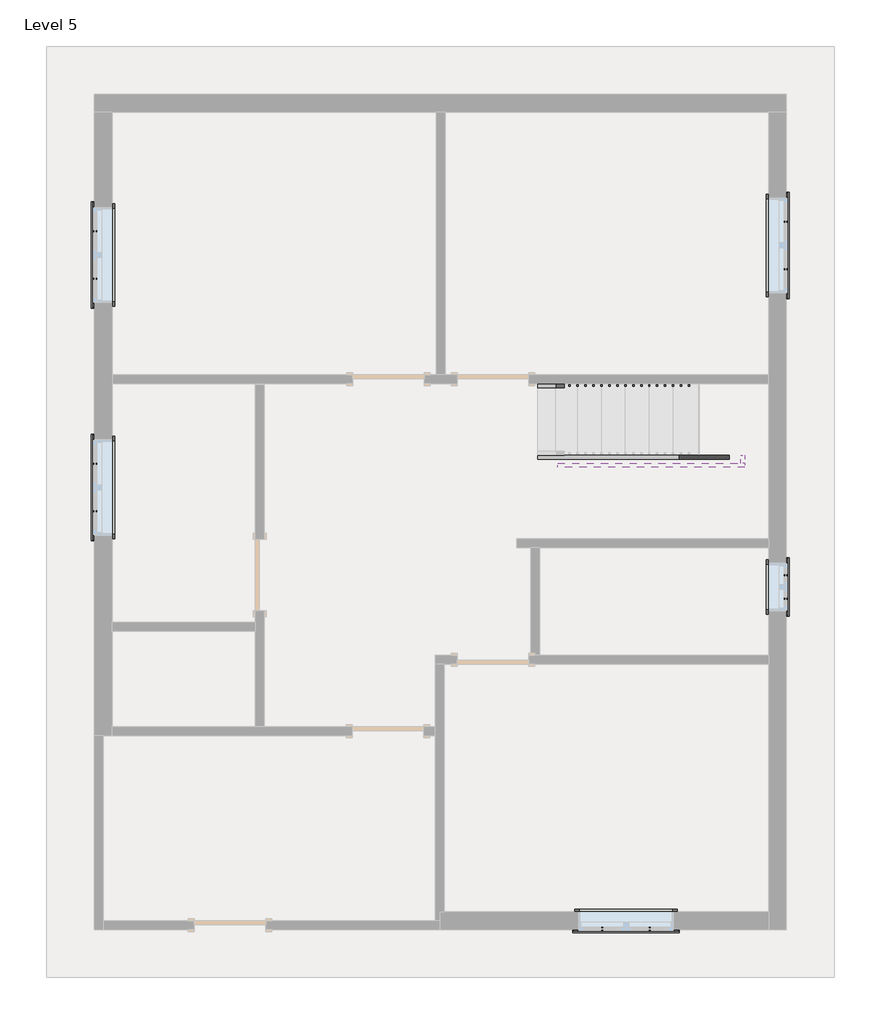
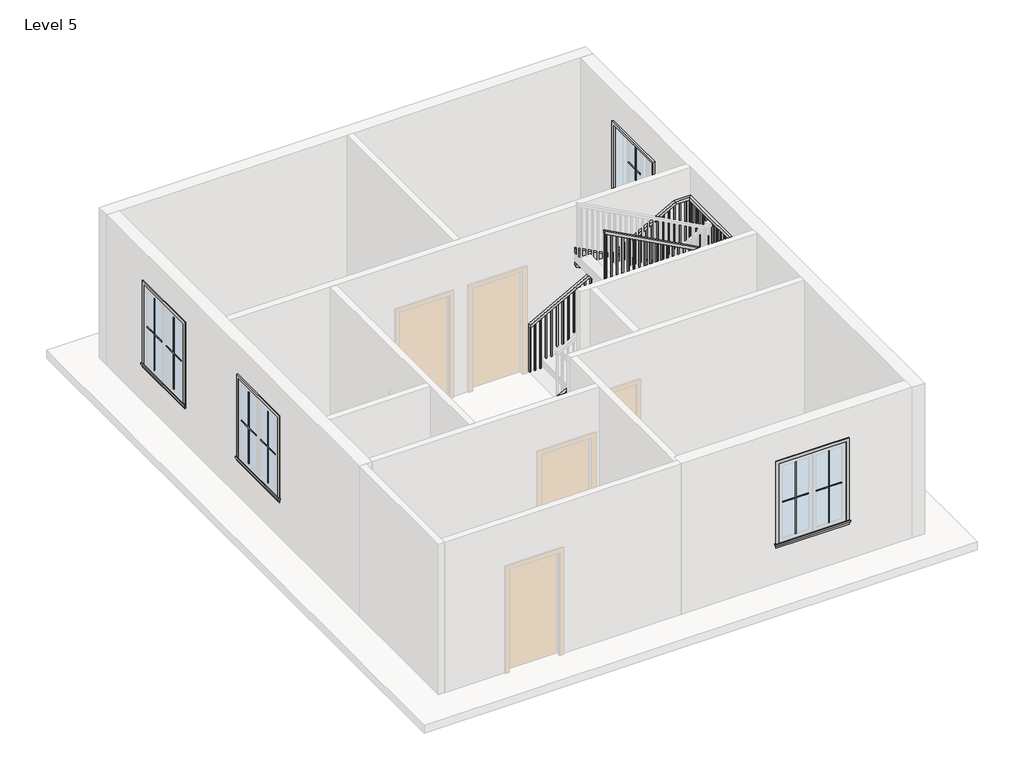
# One storey, part 2 of 2: 20 proxies, 3 members, 1 railing.
"""IFC4 building model written with IfcOpenShell, lengths in millimetres."""

from ifc_helpers import new_model, si_unit, frame, origin, place, context, project, spatial, polyline, outline, extrude, faceted_brep, transform, mapped, element, save
from components import muntin_pattern_2x2_muntin_pattern_2x2_6dad3731, muntin_pattern_2x2_muntin_pattern_2x2_a30a3345, muntin_pattern_2x2_muntin_pattern_2x2_53152e2c, muntin_pattern_2x2_muntin_pattern_2x2_e8f3e573, trim_window_exterior_flat_with_sill_92b9b949, trim_window_exterior_flat_with_sill_a665a915, trim_window_interior_flat_picture_frame_3bb882cf, trim_window_interior_flat_picture_frame_d485c387

model = new_model("IFC4")

# Units and contexts
model_context = context("Model", 3, world=origin())
ifc_project = project(units=[si_unit("LENGTHUNIT", "METRE", prefix="MILLI")], contexts=[model_context])

# Site, building, storey
site = spatial("IfcSite", under=ifc_project)
building = spatial("IfcBuilding", under=site)
storey = spatial("IfcBuildingStorey", under=building, Name="Level 5", Elevation=12192.0)

# Proxies
placement = place(None, origin())
muntin_pattern_2x2_muntin_pattern_2x2_shape = muntin_pattern_2x2_muntin_pattern_2x2_6dad3731(model_context)
element("IfcBuildingElementProxy", 1, Name="Muntin Pattern_2x2 : Muntin Pattern_2x2", ObjectType="Muntin Pattern_2x2 : Muntin Pattern_2x2", at=placement, inside=storey, context=model_context, shape_type="MappedRepresentation", body=[
    mapped(muntin_pattern_2x2_muntin_pattern_2x2_shape, transform((10003.63125, 2232.025, 13176.25), x_axis=(-1.0, 0.0, 0.0), y_axis=(0.0, -1.0, 0.0), z_axis=(0.0, 0.0, 1.0))),
])
element("IfcBuildingElementProxy", 2, Name="Muntin Pattern_2x2 : Muntin Pattern_2x2", ObjectType="Muntin Pattern_2x2 : Muntin Pattern_2x2", at=placement, inside=storey, context=model_context, shape_type="MappedRepresentation", body=[
    mapped(muntin_pattern_2x2_muntin_pattern_2x2_shape, transform((2917.825, 7567.6125, 13176.25), x_axis=(0.0, 1.0, 0.0), y_axis=(-1.0, 0.0, 0.0), z_axis=(0.0, 0.0, 1.0))),
])
element("IfcBuildingElementProxy", 3, Name="Muntin Pattern_2x2 : Muntin Pattern_2x2", ObjectType="Muntin Pattern_2x2 : Muntin Pattern_2x2", at=placement, inside=storey, context=model_context, shape_type="MappedRepresentation", body=[
    mapped(muntin_pattern_2x2_muntin_pattern_2x2_shape, transform((2917.825, 10536.2375, 13176.25), x_axis=(0.0, 1.0, 0.0), y_axis=(-1.0, 0.0, 0.0), z_axis=(0.0, 0.0, 1.0))),
])
element("IfcBuildingElementProxy", 4, Name="Muntin Pattern_2x2 : Muntin Pattern_2x2", ObjectType="Muntin Pattern_2x2 : Muntin Pattern_2x2", at=placement, inside=storey, context=model_context, shape_type="MappedRepresentation", body=[
    mapped(muntin_pattern_2x2_muntin_pattern_2x2_shape, transform((11737.975, 11264.9, 13176.25), x_axis=(0.0, -1.0, 0.0), y_axis=(1.0, 0.0, 0.0), z_axis=(0.0, 0.0, 1.0))),
])
muntin_pattern_2x2_muntin_pattern_2x2_2_shape = muntin_pattern_2x2_muntin_pattern_2x2_a30a3345(model_context)
element("IfcBuildingElementProxy", 5, Name="Muntin Pattern_2x2 : Muntin Pattern_2x2", ObjectType="Muntin Pattern_2x2 : Muntin Pattern_2x2", at=placement, inside=storey, context=model_context, shape_type="MappedRepresentation", body=[
    mapped(muntin_pattern_2x2_muntin_pattern_2x2_2_shape, transform((9397.20625, 2232.025, 13176.25), x_axis=(1.0, 0.0, 0.0), y_axis=(0.0, 1.0, 0.0), z_axis=(0.0, 0.0, 1.0))),
])
element("IfcBuildingElementProxy", 6, Name="Muntin Pattern_2x2 : Muntin Pattern_2x2", ObjectType="Muntin Pattern_2x2 : Muntin Pattern_2x2", at=placement, inside=storey, context=model_context, shape_type="MappedRepresentation", body=[
    mapped(muntin_pattern_2x2_muntin_pattern_2x2_2_shape, transform((2917.825, 8174.0375, 13176.25), x_axis=(0.0, -1.0, 0.0), y_axis=(1.0, 0.0, 0.0), z_axis=(0.0, 0.0, 1.0))),
])
element("IfcBuildingElementProxy", 7, Name="Muntin Pattern_2x2 : Muntin Pattern_2x2", ObjectType="Muntin Pattern_2x2 : Muntin Pattern_2x2", at=placement, inside=storey, context=model_context, shape_type="MappedRepresentation", body=[
    mapped(muntin_pattern_2x2_muntin_pattern_2x2_2_shape, transform((2917.825, 11142.6625, 13176.25), x_axis=(0.0, -1.0, 0.0), y_axis=(1.0, 0.0, 0.0), z_axis=(0.0, 0.0, 1.0))),
])
element("IfcBuildingElementProxy", 8, Name="Muntin Pattern_2x2 : Muntin Pattern_2x2", ObjectType="Muntin Pattern_2x2 : Muntin Pattern_2x2", at=placement, inside=storey, context=model_context, shape_type="MappedRepresentation", body=[
    mapped(muntin_pattern_2x2_muntin_pattern_2x2_2_shape, transform((11737.975, 10658.475, 13176.25), x_axis=(0.0, 1.0, 0.0), y_axis=(-1.0, 0.0, 0.0), z_axis=(0.0, 0.0, 1.0))),
])
muntin_pattern_2x2_muntin_pattern_2x2_3_shape = muntin_pattern_2x2_muntin_pattern_2x2_53152e2c(model_context)
element("IfcBuildingElementProxy", 9, Name="Muntin Pattern_2x2 : Muntin Pattern_2x2", ObjectType="Muntin Pattern_2x2 : Muntin Pattern_2x2", at=placement, inside=storey, context=model_context, shape_type="MappedRepresentation", body=[
    mapped(muntin_pattern_2x2_muntin_pattern_2x2_3_shape, transform((11737.975, 6748.4625, 13176.25), x_axis=(0.0, -1.0, 0.0), y_axis=(1.0, 0.0, 0.0), z_axis=(0.0, 0.0, 1.0))),
])
muntin_pattern_2x2_muntin_pattern_2x2_4_shape = muntin_pattern_2x2_muntin_pattern_2x2_e8f3e573(model_context)
element("IfcBuildingElementProxy", 10, Name="Muntin Pattern_2x2 : Muntin Pattern_2x2", ObjectType="Muntin Pattern_2x2 : Muntin Pattern_2x2", at=placement, inside=storey, context=model_context, shape_type="MappedRepresentation", body=[
    mapped(muntin_pattern_2x2_muntin_pattern_2x2_4_shape, transform((11737.975, 6446.8375, 13176.25), x_axis=(0.0, 1.0, 0.0), y_axis=(-1.0, 0.0, 0.0), z_axis=(0.0, 0.0, 1.0))),
])
trim_window_exterior_flat_with_sill_shape = trim_window_exterior_flat_with_sill_92b9b949(model_context)
element("IfcBuildingElementProxy", 11, Name="Trim-Window-Exterior-Flat : with Sill", ObjectType="Trim-Window-Exterior-Flat : with Sill", at=placement, inside=storey, context=model_context, shape_type="MappedRepresentation", body=[
    mapped(trim_window_exterior_flat_with_sill_shape, transform((9700.41875, 2222.5, 14630.4), x_axis=(1.0, 0.0, 0.0), y_axis=(0.0, 0.0, 1.0), z_axis=(0.0, -1.0, 0.0))),
])
element("IfcBuildingElementProxy", 12, Name="Trim-Window-Exterior-Flat : with Sill", ObjectType="Trim-Window-Exterior-Flat : with Sill", at=placement, inside=storey, context=model_context, shape_type="MappedRepresentation", body=[
    mapped(trim_window_exterior_flat_with_sill_shape, transform((2908.3, 7870.825, 14630.4), x_axis=(0.0, -1.0, 0.0), y_axis=(0.0, 0.0, 1.0), z_axis=(-1.0, 0.0, 0.0))),
])
element("IfcBuildingElementProxy", 13, Name="Trim-Window-Exterior-Flat : with Sill", ObjectType="Trim-Window-Exterior-Flat : with Sill", at=placement, inside=storey, context=model_context, shape_type="MappedRepresentation", body=[
    mapped(trim_window_exterior_flat_with_sill_shape, transform((2908.3, 10839.45, 14630.4), x_axis=(0.0, -1.0, 0.0), y_axis=(0.0, 0.0, 1.0), z_axis=(-1.0, 0.0, 0.0))),
])
element("IfcBuildingElementProxy", 14, Name="Trim-Window-Exterior-Flat : with Sill", ObjectType="Trim-Window-Exterior-Flat : with Sill", at=placement, inside=storey, context=model_context, shape_type="MappedRepresentation", body=[
    mapped(trim_window_exterior_flat_with_sill_shape, transform((11747.5, 10961.6875, 14630.4), x_axis=(0.0, 1.0, 0.0), y_axis=(0.0, 0.0, 1.0), z_axis=(1.0, 0.0, 0.0))),
])
trim_window_exterior_flat_with_sill_2_shape = trim_window_exterior_flat_with_sill_a665a915(model_context)
element("IfcBuildingElementProxy", 15, Name="Trim-Window-Exterior-Flat : with Sill", ObjectType="Trim-Window-Exterior-Flat : with Sill", at=placement, inside=storey, context=model_context, shape_type="MappedRepresentation", body=[
    mapped(trim_window_exterior_flat_with_sill_2_shape, transform((11747.5, 6597.65, 14020.8), x_axis=(0.0, 1.0, 0.0), y_axis=(0.0, 0.0, 1.0), z_axis=(1.0, 0.0, 0.0))),
])
trim_window_interior_flat_picture_frame_shape = trim_window_interior_flat_picture_frame_3bb882cf(model_context)
element("IfcBuildingElementProxy", 16, Name="Trim-Window-Interior-Flat : Picture Frame", ObjectType="Trim-Window-Interior-Flat : Picture Frame", at=placement, inside=storey, context=model_context, shape_type="MappedRepresentation", body=[
    mapped(trim_window_interior_flat_picture_frame_shape, transform((9700.41875, 2451.1, 14630.4), x_axis=(-1.0, 0.0, 0.0), y_axis=(0.0, 0.0, 1.0), z_axis=(0.0, 1.0, 0.0))),
])
element("IfcBuildingElementProxy", 17, Name="Trim-Window-Interior-Flat : Picture Frame", ObjectType="Trim-Window-Interior-Flat : Picture Frame", at=placement, inside=storey, context=model_context, shape_type="MappedRepresentation", body=[
    mapped(trim_window_interior_flat_picture_frame_shape, transform((3136.9, 7870.825, 14630.4), x_axis=(0.0, 1.0, 0.0), y_axis=(0.0, 0.0, 1.0), z_axis=(1.0, 0.0, 0.0))),
])
element("IfcBuildingElementProxy", 18, Name="Trim-Window-Interior-Flat : Picture Frame", ObjectType="Trim-Window-Interior-Flat : Picture Frame", at=placement, inside=storey, context=model_context, shape_type="MappedRepresentation", body=[
    mapped(trim_window_interior_flat_picture_frame_shape, transform((3136.9, 10839.45, 14630.4), x_axis=(0.0, 1.0, 0.0), y_axis=(0.0, 0.0, 1.0), z_axis=(1.0, 0.0, 0.0))),
])
element("IfcBuildingElementProxy", 19, Name="Trim-Window-Interior-Flat : Picture Frame", ObjectType="Trim-Window-Interior-Flat : Picture Frame", at=placement, inside=storey, context=model_context, shape_type="MappedRepresentation", body=[
    mapped(trim_window_interior_flat_picture_frame_shape, transform((11518.9, 10961.6875, 14630.4), x_axis=(0.0, -1.0, 0.0), y_axis=(0.0, 0.0, 1.0), z_axis=(-1.0, 0.0, 0.0))),
])
trim_window_interior_flat_picture_frame_2_shape = trim_window_interior_flat_picture_frame_d485c387(model_context)
element("IfcBuildingElementProxy", 20, Name="Trim-Window-Interior-Flat : Picture Frame", ObjectType="Trim-Window-Interior-Flat : Picture Frame", at=placement, inside=storey, context=model_context, shape_type="MappedRepresentation", body=[
    mapped(trim_window_interior_flat_picture_frame_2_shape, transform((11518.9, 6597.65, 14020.8), x_axis=(0.0, -1.0, 0.0), y_axis=(0.0, 0.0, 1.0), z_axis=(-1.0, 0.0, 0.0))),
])

# Members
element("IfcMember", 21, ObjectType="Stringer - 2\" Width", at=placement, inside=storey, context=model_context, shape_type="SweptSolid", body=[
    extrude(outline(polyline([(12436.4581083, 8572.5), (12192.0, 8572.5), (12192.0, 8761.9689927), (13469.1621978, 11163.3), (13814.3905183, 11163.3), (12436.4581083, 8572.5)])), frame((0.0, 8229.6, 0.0), z_axis=(0.0, 1.0, 0.0), x_axis=(0.0, 0.0, 1.0)), (0.0, 0.0, 1.0), 50.8),
])
element("IfcMember", 22, ObjectType="Stringer - 2\" Width", at=placement, inside=storey, context=model_context, shape_type="SweptSolid", body=[
    extrude(outline(polyline([(11163.3, 8280.4), (11214.1, 8280.4), (11214.1, 8178.8), (11163.3, 8178.8), (11163.3, 8280.4)])), frame((0.0, 0.0, 13567.6105263), z_axis=(0.0, 0.0, 1.0), x_axis=(1.0, 0.0, 0.0)), (0.0, 0.0, 1.0), 304.8),
])
element("IfcMember", 23, ObjectType="Stringer - 2\" Width", at=placement, inside=storey, context=model_context, shape_type="SweptSolid", body=[
    extrude(outline(polyline([(13656.9419568, 11214.1), (14001.380564, 11214.1), (15258.012143, 8826.5), (14913.5735358, 8826.5), (13656.9419568, 11214.1)])), frame((0.0, 8128.0, 0.0), z_axis=(0.0, 1.0, 0.0), x_axis=(0.0, 0.0, 1.0)), (0.0, 0.0, 1.0), 50.8),
])

# Railing
element("IfcRailing", 24, ObjectType="Handrail - Rectangular", at=placement, inside=storey, context=model_context, shape_type="SolidModel", body=[
    faceted_brep([(8572.5, 9194.8, 13266.8210526), (8572.5, 9194.8, 13208.9285199), (8572.5, 9144.0, 13208.9285199), (8572.5, 9144.0, 13266.8210526), (11214.1, 9194.8, 14710.6105263), (11227.076708, 9194.8, 14659.8105263), (11227.076708, 9144.0, 14659.8105263), (11214.1, 9144.0, 14710.6105263), (11518.9, 9194.8, 14710.6105263), (11518.9, 9194.8, 14659.8105263), (11468.1, 9144.0, 14659.8105263), (11468.1, 9144.0, 14710.6105263), (11518.9, 7340.6, 14710.6105263), (11518.9, 7289.8, 14659.8105263), (11468.1, 7289.8, 14659.8105263), (11468.1, 7340.6, 14710.6105263), (11518.9, 7340.6, 14775.4615901), (11518.9, 7289.8, 14724.6615901), (11468.1, 7289.8, 14724.6615901), (11468.1, 7340.6, 14775.4615901), (11518.9, 7213.6, 14775.4615901), (11518.9, 7213.6, 14724.6615901), (11468.1, 7264.4, 14724.6615901), (11468.1, 7264.4, 14775.4615901), (11391.9, 7213.6, 14775.4615901), (11379.1122768, 7213.6, 14724.6615901), (11379.1122768, 7264.4, 14724.6615901), (11391.9, 7264.4, 14775.4615901), (8826.5, 7213.6, 16154.4), (8826.5, 7264.4, 16154.4), (8826.5, 7264.4, 16096.7264198), (8826.5, 7213.6, 16096.7264198)], [[[0, 1, 2, 3]], [[1, 0, 4, 5]], [[2, 1, 5, 6]], [[3, 2, 6, 7]], [[0, 3, 7, 4]], [[5, 4, 8, 9]], [[6, 5, 9, 10]], [[7, 6, 10, 11]], [[4, 7, 11, 8]], [[9, 8, 12, 13]], [[10, 9, 13, 14]], [[11, 10, 14, 15]], [[8, 11, 15, 12]], [[13, 12, 16, 17]], [[14, 13, 17, 18]], [[15, 14, 18, 19]], [[12, 15, 19, 16]], [[17, 16, 20, 21]], [[18, 17, 21, 22]], [[19, 18, 22, 23]], [[16, 19, 23, 20]], [[21, 20, 24, 25]], [[22, 21, 25, 26]], [[23, 22, 26, 27]], [[20, 23, 27, 24]], [[28, 29, 30, 31]], [[25, 24, 28, 31]], [[26, 25, 31, 30]], [[27, 26, 30, 29]], [[24, 27, 29, 28]]]),
    extrude(outline(polyline([(16088.193385, 8842.375), (15079.5789474, 8842.375), (15079.5789474, 8861.425), (16077.9537434, 8861.425), (16088.193385, 8842.375)])), frame((0.0, 7229.475, 0.0), z_axis=(0.0, 1.0, 0.0), x_axis=(0.0, 0.0, 1.0)), (0.0, 0.0, 1.0), 19.05),
    extrude(outline(polyline([(16033.5819629, 8943.975), (15079.5789474, 8943.975), (15079.5789474, 8963.025), (16023.3423212, 8963.025), (16033.5819629, 8943.975)])), frame((0.0, 7229.475, 0.0), z_axis=(0.0, 1.0, 0.0), x_axis=(0.0, 0.0, 1.0)), (0.0, 0.0, 1.0), 19.05),
    extrude(outline(polyline([(15978.9705407, 9045.575), (15079.5789474, 9045.575), (15079.5789474, 9064.625), (15968.730899, 9064.625), (15978.9705407, 9045.575)])), frame((0.0, 7229.475, 0.0), z_axis=(0.0, 1.0, 0.0), x_axis=(0.0, 0.0, 1.0)), (0.0, 0.0, 1.0), 19.05),
    extrude(outline(polyline([(15924.3591185, 9147.175), (14919.1578947, 9147.175), (14919.1578947, 9166.225), (15914.1194769, 9166.225), (15924.3591185, 9147.175)])), frame((0.0, 7229.475, 0.0), z_axis=(0.0, 1.0, 0.0), x_axis=(0.0, 0.0, 1.0)), (0.0, 0.0, 1.0), 19.05),
    extrude(outline(polyline([(15869.7476964, 9248.775), (14919.1578947, 9248.775), (14919.1578947, 9267.825), (15859.5080547, 9267.825), (15869.7476964, 9248.775)])), frame((0.0, 7229.475, 0.0), z_axis=(0.0, 1.0, 0.0), x_axis=(0.0, 0.0, 1.0)), (0.0, 0.0, 1.0), 19.05),
    extrude(outline(polyline([(15815.1362742, 9350.375), (14919.1578947, 9350.375), (14919.1578947, 9369.425), (15804.8966325, 9369.425), (15815.1362742, 9350.375)])), frame((0.0, 7229.475, 0.0), z_axis=(0.0, 1.0, 0.0), x_axis=(0.0, 0.0, 1.0)), (0.0, 0.0, 1.0), 19.05),
    extrude(outline(polyline([(15760.524852, 9451.975), (14758.7368421, 9451.975), (14758.7368421, 9471.025), (15750.2852104, 9471.025), (15760.524852, 9451.975)])), frame((0.0, 7229.475, 0.0), z_axis=(0.0, 1.0, 0.0), x_axis=(0.0, 0.0, 1.0)), (0.0, 0.0, 1.0), 19.05),
    extrude(outline(polyline([(15705.9134298, 9553.575), (14758.7368421, 9553.575), (14758.7368421, 9572.625), (15695.6737882, 9572.625), (15705.9134298, 9553.575)])), frame((0.0, 7229.475, 0.0), z_axis=(0.0, 1.0, 0.0), x_axis=(0.0, 0.0, 1.0)), (0.0, 0.0, 1.0), 19.05),
    extrude(outline(polyline([(15651.3004835, 9655.175), (14758.7368421, 9655.175), (14758.7368421, 9674.225), (15640.8885402, 9674.225), (15651.3004835, 9655.175)])), frame((0.0, 7229.475, 0.0), z_axis=(0.0, 1.0, 0.0), x_axis=(0.0, 0.0, 1.0)), (0.0, 0.0, 1.0), 19.05),
    extrude(outline(polyline([(15596.6905855, 9756.775), (14598.3157895, 9756.775), (14598.3157895, 9775.825), (15586.4509438, 9775.825), (15596.6905855, 9756.775)])), frame((0.0, 7229.475, 0.0), z_axis=(0.0, 1.0, 0.0), x_axis=(0.0, 0.0, 1.0)), (0.0, 0.0, 1.0), 19.05),
    extrude(outline(polyline([(15542.0791633, 9858.375), (14598.3157895, 9858.375), (14598.3157895, 9877.425), (15531.8395217, 9877.425), (15542.0791633, 9858.375)])), frame((0.0, 7229.475, 0.0), z_axis=(0.0, 1.0, 0.0), x_axis=(0.0, 0.0, 1.0)), (0.0, 0.0, 1.0), 19.05),
    extrude(outline(polyline([(15487.4677411, 9959.975), (14598.3157895, 9959.975), (14598.3157895, 9979.025), (15477.2280995, 9979.025), (15487.4677411, 9959.975)])), frame((0.0, 7229.475, 0.0), z_axis=(0.0, 1.0, 0.0), x_axis=(0.0, 0.0, 1.0)), (0.0, 0.0, 1.0), 19.05),
    extrude(outline(polyline([(15432.856319, 10061.575), (14437.8947368, 10061.575), (14437.8947368, 10080.625), (15422.6166773, 10080.625), (15432.856319, 10061.575)])), frame((0.0, 7229.475, 0.0), z_axis=(0.0, 1.0, 0.0), x_axis=(0.0, 0.0, 1.0)), (0.0, 0.0, 1.0), 19.05),
    extrude(outline(polyline([(15378.2448968, 10163.175), (14437.8947368, 10163.175), (14437.8947368, 10182.225), (15368.0052551, 10182.225), (15378.2448968, 10163.175)])), frame((0.0, 7229.475, 0.0), z_axis=(0.0, 1.0, 0.0), x_axis=(0.0, 0.0, 1.0)), (0.0, 0.0, 1.0), 19.05),
    extrude(outline(polyline([(15323.6334746, 10264.775), (14437.8947368, 10264.775), (14437.8947368, 10283.825), (15313.393833, 10283.825), (15323.6334746, 10264.775)])), frame((0.0, 7229.475, 0.0), z_axis=(0.0, 1.0, 0.0), x_axis=(0.0, 0.0, 1.0)), (0.0, 0.0, 1.0), 19.05),
    extrude(outline(polyline([(15269.0220525, 10366.375), (14277.4736842, 10366.375), (14277.4736842, 10385.425), (15258.7824108, 10385.425), (15269.0220525, 10366.375)])), frame((0.0, 7229.475, 0.0), z_axis=(0.0, 1.0, 0.0), x_axis=(0.0, 0.0, 1.0)), (0.0, 0.0, 1.0), 19.05),
    extrude(outline(polyline([(15214.4106303, 10467.975), (14277.4736842, 10467.975), (14277.4736842, 10487.025), (15204.1709886, 10487.025), (15214.4106303, 10467.975)])), frame((0.0, 7229.475, 0.0), z_axis=(0.0, 1.0, 0.0), x_axis=(0.0, 0.0, 1.0)), (0.0, 0.0, 1.0), 19.05),
    extrude(outline(polyline([(15159.7992081, 10569.575), (14277.4736842, 10569.575), (14277.4736842, 10588.625), (15149.5595665, 10588.625), (15159.7992081, 10569.575)])), frame((0.0, 7229.475, 0.0), z_axis=(0.0, 1.0, 0.0), x_axis=(0.0, 0.0, 1.0)), (0.0, 0.0, 1.0), 19.05),
    extrude(outline(polyline([(15105.1877859, 10671.175), (14117.0526316, 10671.175), (14117.0526316, 10690.225), (15094.9481443, 10690.225), (15105.1877859, 10671.175)])), frame((0.0, 7229.475, 0.0), z_axis=(0.0, 1.0, 0.0), x_axis=(0.0, 0.0, 1.0)), (0.0, 0.0, 1.0), 19.05),
    extrude(outline(polyline([(15050.5763638, 10772.775), (14117.0526316, 10772.775), (14117.0526316, 10791.825), (15040.3367221, 10791.825), (15050.5763638, 10772.775)])), frame((0.0, 7229.475, 0.0), z_axis=(0.0, 1.0, 0.0), x_axis=(0.0, 0.0, 1.0)), (0.0, 0.0, 1.0), 19.05),
    extrude(outline(polyline([(14995.9649416, 10874.375), (14117.0526316, 10874.375), (14117.0526316, 10893.425), (14985.7252999, 10893.425), (14995.9649416, 10874.375)])), frame((0.0, 7229.475, 0.0), z_axis=(0.0, 1.0, 0.0), x_axis=(0.0, 0.0, 1.0)), (0.0, 0.0, 1.0), 19.05),
    extrude(outline(polyline([(14941.3535194, 10975.975), (13956.6315789, 10975.975), (13956.6315789, 10995.025), (14931.1138778, 10995.025), (14941.3535194, 10975.975)])), frame((0.0, 7229.475, 0.0), z_axis=(0.0, 1.0, 0.0), x_axis=(0.0, 0.0, 1.0)), (0.0, 0.0, 1.0), 19.05),
    extrude(outline(polyline([(14886.7420972, 11077.575), (13956.6315789, 11077.575), (13956.6315789, 11096.625), (14876.5024556, 11096.625), (14886.7420972, 11077.575)])), frame((0.0, 7229.475, 0.0), z_axis=(0.0, 1.0, 0.0), x_axis=(0.0, 0.0, 1.0)), (0.0, 0.0, 1.0), 19.05),
    extrude(outline(polyline([(14832.1306751, 11179.175), (13956.6315789, 11179.175), (13956.6315789, 11198.225), (14821.8910334, 11198.225), (14832.1306751, 11179.175)])), frame((0.0, 7229.475, 0.0), z_axis=(0.0, 1.0, 0.0), x_axis=(0.0, 0.0, 1.0)), (0.0, 0.0, 1.0), 19.05),
    extrude(outline(polyline([(14777.5192529, 11280.775), (13796.2105263, 11280.775), (13796.2105263, 11299.825), (14767.2796112, 11299.825), (14777.5192529, 11280.775)])), frame((0.0, 7229.475, 0.0), z_axis=(0.0, 1.0, 0.0), x_axis=(0.0, 0.0, 1.0)), (0.0, 0.0, 1.0), 19.05),
    extrude(outline(polyline([(14722.9078307, 11382.375), (13796.2105263, 11382.375), (13796.2105263, 11401.425), (14712.6681891, 11401.425), (14722.9078307, 11382.375)])), frame((0.0, 7229.475, 0.0), z_axis=(0.0, 1.0, 0.0), x_axis=(0.0, 0.0, 1.0)), (0.0, 0.0, 1.0), 19.05),
    extrude(outline(polyline([(11503.025, 7350.125), (11503.025, 7331.075), (11483.975, 7331.075), (11483.975, 7350.125), (11503.025, 7350.125)])), frame((0.0, 0.0, 13796.2105263), z_axis=(0.0, 0.0, 1.0), x_axis=(1.0, 0.0, 0.0)), (0.0, 0.0, 1.0), 863.6),
    extrude(outline(polyline([(11503.025, 7451.725), (11503.025, 7432.675), (11483.975, 7432.675), (11483.975, 7451.725), (11503.025, 7451.725)])), frame((0.0, 0.0, 13796.2105263), z_axis=(0.0, 0.0, 1.0), x_axis=(1.0, 0.0, 0.0)), (0.0, 0.0, 1.0), 863.6),
    extrude(outline(polyline([(11503.025, 7553.325), (11503.025, 7534.275), (11483.975, 7534.275), (11483.975, 7553.325), (11503.025, 7553.325)])), frame((0.0, 0.0, 13796.2105263), z_axis=(0.0, 0.0, 1.0), x_axis=(1.0, 0.0, 0.0)), (0.0, 0.0, 1.0), 863.6),
    extrude(outline(polyline([(11503.025, 7654.925), (11503.025, 7635.875), (11483.975, 7635.875), (11483.975, 7654.925), (11503.025, 7654.925)])), frame((0.0, 0.0, 13796.2105263), z_axis=(0.0, 0.0, 1.0), x_axis=(1.0, 0.0, 0.0)), (0.0, 0.0, 1.0), 863.6),
    extrude(outline(polyline([(11503.025, 7756.525), (11503.025, 7737.475), (11483.975, 7737.475), (11483.975, 7756.525), (11503.025, 7756.525)])), frame((0.0, 0.0, 13796.2105263), z_axis=(0.0, 0.0, 1.0), x_axis=(1.0, 0.0, 0.0)), (0.0, 0.0, 1.0), 863.6),
    extrude(outline(polyline([(11503.025, 7858.125), (11503.025, 7839.075), (11483.975, 7839.075), (11483.975, 7858.125), (11503.025, 7858.125)])), frame((0.0, 0.0, 13796.2105263), z_axis=(0.0, 0.0, 1.0), x_axis=(1.0, 0.0, 0.0)), (0.0, 0.0, 1.0), 863.6),
    extrude(outline(polyline([(11503.025, 7959.725), (11503.025, 7940.675), (11483.975, 7940.675), (11483.975, 7959.725), (11503.025, 7959.725)])), frame((0.0, 0.0, 13796.2105263), z_axis=(0.0, 0.0, 1.0), x_axis=(1.0, 0.0, 0.0)), (0.0, 0.0, 1.0), 863.6),
    extrude(outline(polyline([(11503.025, 8061.325), (11503.025, 8042.275), (11483.975, 8042.275), (11483.975, 8061.325), (11503.025, 8061.325)])), frame((0.0, 0.0, 13796.2105263), z_axis=(0.0, 0.0, 1.0), x_axis=(1.0, 0.0, 0.0)), (0.0, 0.0, 1.0), 863.6),
    extrude(outline(polyline([(11503.025, 8162.925), (11503.025, 8143.875), (11483.975, 8143.875), (11483.975, 8162.925), (11503.025, 8162.925)])), frame((0.0, 0.0, 13796.2105263), z_axis=(0.0, 0.0, 1.0), x_axis=(1.0, 0.0, 0.0)), (0.0, 0.0, 1.0), 863.6),
    extrude(outline(polyline([(11503.025, 8264.525), (11503.025, 8245.475), (11483.975, 8245.475), (11483.975, 8264.525), (11503.025, 8264.525)])), frame((0.0, 0.0, 13796.2105263), z_axis=(0.0, 0.0, 1.0), x_axis=(1.0, 0.0, 0.0)), (0.0, 0.0, 1.0), 863.6),
    extrude(outline(polyline([(11503.025, 8366.125), (11503.025, 8347.075), (11483.975, 8347.075), (11483.975, 8366.125), (11503.025, 8366.125)])), frame((0.0, 0.0, 13796.2105263), z_axis=(0.0, 0.0, 1.0), x_axis=(1.0, 0.0, 0.0)), (0.0, 0.0, 1.0), 863.6),
    extrude(outline(polyline([(11503.025, 8467.725), (11503.025, 8448.675), (11483.975, 8448.675), (11483.975, 8467.725), (11503.025, 8467.725)])), frame((0.0, 0.0, 13796.2105263), z_axis=(0.0, 0.0, 1.0), x_axis=(1.0, 0.0, 0.0)), (0.0, 0.0, 1.0), 863.6),
    extrude(outline(polyline([(11503.025, 8569.325), (11503.025, 8550.275), (11483.975, 8550.275), (11483.975, 8569.325), (11503.025, 8569.325)])), frame((0.0, 0.0, 13796.2105263), z_axis=(0.0, 0.0, 1.0), x_axis=(1.0, 0.0, 0.0)), (0.0, 0.0, 1.0), 863.6),
    extrude(outline(polyline([(11503.025, 8670.925), (11503.025, 8651.875), (11483.975, 8651.875), (11483.975, 8670.925), (11503.025, 8670.925)])), frame((0.0, 0.0, 13796.2105263), z_axis=(0.0, 0.0, 1.0), x_axis=(1.0, 0.0, 0.0)), (0.0, 0.0, 1.0), 863.6),
    extrude(outline(polyline([(11503.025, 8772.525), (11503.025, 8753.475), (11483.975, 8753.475), (11483.975, 8772.525), (11503.025, 8772.525)])), frame((0.0, 0.0, 13796.2105263), z_axis=(0.0, 0.0, 1.0), x_axis=(1.0, 0.0, 0.0)), (0.0, 0.0, 1.0), 863.6),
    extrude(outline(polyline([(11503.025, 8874.125), (11503.025, 8855.075), (11483.975, 8855.075), (11483.975, 8874.125), (11503.025, 8874.125)])), frame((0.0, 0.0, 13796.2105263), z_axis=(0.0, 0.0, 1.0), x_axis=(1.0, 0.0, 0.0)), (0.0, 0.0, 1.0), 863.6),
    extrude(outline(polyline([(11503.025, 8975.725), (11503.025, 8956.675), (11483.975, 8956.675), (11483.975, 8975.725), (11503.025, 8975.725)])), frame((0.0, 0.0, 13796.2105263), z_axis=(0.0, 0.0, 1.0), x_axis=(1.0, 0.0, 0.0)), (0.0, 0.0, 1.0), 863.6),
    extrude(outline(polyline([(11503.025, 9077.325), (11503.025, 9058.275), (11483.975, 9058.275), (11483.975, 9077.325), (11503.025, 9077.325)])), frame((0.0, 0.0, 13796.2105263), z_axis=(0.0, 0.0, 1.0), x_axis=(1.0, 0.0, 0.0)), (0.0, 0.0, 1.0), 863.6),
    extrude(outline(polyline([(11407.775, 9178.925), (11426.825, 9178.925), (11426.825, 9159.875), (11407.775, 9159.875), (11407.775, 9178.925)])), frame((0.0, 0.0, 13796.2105263), z_axis=(0.0, 0.0, 1.0), x_axis=(1.0, 0.0, 0.0)), (0.0, 0.0, 1.0), 863.6),
    extrude(outline(polyline([(11306.175, 9178.925), (11325.225, 9178.925), (11325.225, 9159.875), (11306.175, 9159.875), (11306.175, 9178.925)])), frame((0.0, 0.0, 13796.2105263), z_axis=(0.0, 0.0, 1.0), x_axis=(1.0, 0.0, 0.0)), (0.0, 0.0, 1.0), 863.6),
    extrude(outline(polyline([(14647.512022, 11204.575), (13796.2105263, 11204.575), (13796.2105263, 11223.625), (14657.9239653, 11223.625), (14647.512022, 11204.575)])), frame((0.0, 9159.875, 0.0), z_axis=(0.0, 1.0, 0.0), x_axis=(0.0, 0.0, 1.0)), (0.0, 0.0, 1.0), 19.05),
    extrude(outline(polyline([(14591.9816576, 11102.975), (13635.7894737, 11102.975), (13635.7894737, 11122.025), (14602.3936009, 11122.025), (14591.9816576, 11102.975)])), frame((0.0, 9159.875, 0.0), z_axis=(0.0, 1.0, 0.0), x_axis=(0.0, 0.0, 1.0)), (0.0, 0.0, 1.0), 19.05),
    extrude(outline(polyline([(14536.4512932, 11001.375), (13635.7894737, 11001.375), (13635.7894737, 11020.425), (14546.8632365, 11020.425), (14536.4512932, 11001.375)])), frame((0.0, 9159.875, 0.0), z_axis=(0.0, 1.0, 0.0), x_axis=(0.0, 0.0, 1.0)), (0.0, 0.0, 1.0), 19.05),
    extrude(outline(polyline([(14480.9209288, 10899.775), (13635.7894737, 10899.775), (13635.7894737, 10918.825), (14491.3328722, 10918.825), (14480.9209288, 10899.775)])), frame((0.0, 9159.875, 0.0), z_axis=(0.0, 1.0, 0.0), x_axis=(0.0, 0.0, 1.0)), (0.0, 0.0, 1.0), 19.05),
    extrude(outline(polyline([(14425.3905645, 10798.175), (13475.3684211, 10798.175), (13475.3684211, 10817.225), (14435.8025078, 10817.225), (14425.3905645, 10798.175)])), frame((0.0, 9159.875, 0.0), z_axis=(0.0, 1.0, 0.0), x_axis=(0.0, 0.0, 1.0)), (0.0, 0.0, 1.0), 19.05),
    extrude(outline(polyline([(14369.8602001, 10696.575), (13475.3684211, 10696.575), (13475.3684211, 10715.625), (14380.2721434, 10715.625), (14369.8602001, 10696.575)])), frame((0.0, 9159.875, 0.0), z_axis=(0.0, 1.0, 0.0), x_axis=(0.0, 0.0, 1.0)), (0.0, 0.0, 1.0), 19.05),
    extrude(outline(polyline([(14314.3298357, 10594.975), (13475.3684211, 10594.975), (13475.3684211, 10614.025), (14324.741779, 10614.025), (14314.3298357, 10594.975)])), frame((0.0, 9159.875, 0.0), z_axis=(0.0, 1.0, 0.0), x_axis=(0.0, 0.0, 1.0)), (0.0, 0.0, 1.0), 19.05),
    extrude(outline(polyline([(14258.7994714, 10493.375), (13314.9473684, 10493.375), (13314.9473684, 10512.425), (14269.2114147, 10512.425), (14258.7994714, 10493.375)])), frame((0.0, 9159.875, 0.0), z_axis=(0.0, 1.0, 0.0), x_axis=(0.0, 0.0, 1.0)), (0.0, 0.0, 1.0), 19.05),
    extrude(outline(polyline([(14203.269107, 10391.775), (13314.9473684, 10391.775), (13314.9473684, 10410.825), (14213.6810503, 10410.825), (14203.269107, 10391.775)])), frame((0.0, 9159.875, 0.0), z_axis=(0.0, 1.0, 0.0), x_axis=(0.0, 0.0, 1.0)), (0.0, 0.0, 1.0), 19.05),
    extrude(outline(polyline([(14147.7387426, 10290.175), (13314.9473684, 10290.175), (13314.9473684, 10309.225), (14158.1506859, 10309.225), (14147.7387426, 10290.175)])), frame((0.0, 9159.875, 0.0), z_axis=(0.0, 1.0, 0.0), x_axis=(0.0, 0.0, 1.0)), (0.0, 0.0, 1.0), 19.05),
    extrude(outline(polyline([(14092.2083782, 10188.575), (13154.5263158, 10188.575), (13154.5263158, 10207.625), (14102.6203216, 10207.625), (14092.2083782, 10188.575)])), frame((0.0, 9159.875, 0.0), z_axis=(0.0, 1.0, 0.0), x_axis=(0.0, 0.0, 1.0)), (0.0, 0.0, 1.0), 19.05),
    extrude(outline(polyline([(14036.6780139, 10086.975), (13154.5263158, 10086.975), (13154.5263158, 10106.025), (14047.0899572, 10106.025), (14036.6780139, 10086.975)])), frame((0.0, 9159.875, 0.0), z_axis=(0.0, 1.0, 0.0), x_axis=(0.0, 0.0, 1.0)), (0.0, 0.0, 1.0), 19.05),
    extrude(outline(polyline([(13981.1476495, 9985.375), (13154.5263158, 9985.375), (13154.5263158, 10004.425), (13991.5595928, 10004.425), (13981.1476495, 9985.375)])), frame((0.0, 9159.875, 0.0), z_axis=(0.0, 1.0, 0.0), x_axis=(0.0, 0.0, 1.0)), (0.0, 0.0, 1.0), 19.05),
    extrude(outline(polyline([(13925.6172851, 9883.775), (12994.1052632, 9883.775), (12994.1052632, 9902.825), (13936.0292284, 9902.825), (13925.6172851, 9883.775)])), frame((0.0, 9159.875, 0.0), z_axis=(0.0, 1.0, 0.0), x_axis=(0.0, 0.0, 1.0)), (0.0, 0.0, 1.0), 19.05),
    extrude(outline(polyline([(13870.0869207, 9782.175), (12994.1052632, 9782.175), (12994.1052632, 9801.225), (13880.4988641, 9801.225), (13870.0869207, 9782.175)])), frame((0.0, 9159.875, 0.0), z_axis=(0.0, 1.0, 0.0), x_axis=(0.0, 0.0, 1.0)), (0.0, 0.0, 1.0), 19.05),
    extrude(outline(polyline([(13814.5565564, 9680.575), (12994.1052632, 9680.575), (12994.1052632, 9699.625), (13824.9684997, 9699.625), (13814.5565564, 9680.575)])), frame((0.0, 9159.875, 0.0), z_axis=(0.0, 1.0, 0.0), x_axis=(0.0, 0.0, 1.0)), (0.0, 0.0, 1.0), 19.05),
    extrude(outline(polyline([(13759.026192, 9578.975), (12833.6842105, 9578.975), (12833.6842105, 9598.025), (13769.4381353, 9598.025), (13759.026192, 9578.975)])), frame((0.0, 9159.875, 0.0), z_axis=(0.0, 1.0, 0.0), x_axis=(0.0, 0.0, 1.0)), (0.0, 0.0, 1.0), 19.05),
    extrude(outline(polyline([(13703.4958276, 9477.375), (12833.6842105, 9477.375), (12833.6842105, 9496.425), (13713.9077709, 9496.425), (13703.4958276, 9477.375)])), frame((0.0, 9159.875, 0.0), z_axis=(0.0, 1.0, 0.0), x_axis=(0.0, 0.0, 1.0)), (0.0, 0.0, 1.0), 19.05),
    extrude(outline(polyline([(13647.9654633, 9375.775), (12833.6842105, 9375.775), (12833.6842105, 9394.825), (13658.3774066, 9394.825), (13647.9654633, 9375.775)])), frame((0.0, 9159.875, 0.0), z_axis=(0.0, 1.0, 0.0), x_axis=(0.0, 0.0, 1.0)), (0.0, 0.0, 1.0), 19.05),
    extrude(outline(polyline([(13592.4350989, 9274.175), (12673.2631579, 9274.175), (12673.2631579, 9293.225), (13602.8470422, 9293.225), (13592.4350989, 9274.175)])), frame((0.0, 9159.875, 0.0), z_axis=(0.0, 1.0, 0.0), x_axis=(0.0, 0.0, 1.0)), (0.0, 0.0, 1.0), 19.05),
    extrude(outline(polyline([(13536.9047345, 9172.575), (12673.2631579, 9172.575), (12673.2631579, 9191.625), (13547.3166778, 9191.625), (13536.9047345, 9172.575)])), frame((0.0, 9159.875, 0.0), z_axis=(0.0, 1.0, 0.0), x_axis=(0.0, 0.0, 1.0)), (0.0, 0.0, 1.0), 19.05),
    extrude(outline(polyline([(13481.3743701, 9070.975), (12673.2631579, 9070.975), (12673.2631579, 9090.025), (13491.7863135, 9090.025), (13481.3743701, 9070.975)])), frame((0.0, 9159.875, 0.0), z_axis=(0.0, 1.0, 0.0), x_axis=(0.0, 0.0, 1.0)), (0.0, 0.0, 1.0), 19.05),
    extrude(outline(polyline([(13425.8440058, 8969.375), (12512.8421053, 8969.375), (12512.8421053, 8988.425), (13436.2559491, 8988.425), (13425.8440058, 8969.375)])), frame((0.0, 9159.875, 0.0), z_axis=(0.0, 1.0, 0.0), x_axis=(0.0, 0.0, 1.0)), (0.0, 0.0, 1.0), 19.05),
    extrude(outline(polyline([(13370.3136414, 8867.775), (12512.8421053, 8867.775), (12512.8421053, 8886.825), (13380.7255847, 8886.825), (13370.3136414, 8867.775)])), frame((0.0, 9159.875, 0.0), z_axis=(0.0, 1.0, 0.0), x_axis=(0.0, 0.0, 1.0)), (0.0, 0.0, 1.0), 19.05),
    extrude(outline(polyline([(13314.783277, 8766.175), (12352.4210526, 8766.175), (12352.4210526, 8785.225), (13325.1952203, 8785.225), (13314.783277, 8766.175)])), frame((0.0, 9159.875, 0.0), z_axis=(0.0, 1.0, 0.0), x_axis=(0.0, 0.0, 1.0)), (0.0, 0.0, 1.0), 19.05),
    extrude(outline(polyline([(13259.2529126, 8664.575), (12352.4210526, 8664.575), (12352.4210526, 8683.625), (13269.664856, 8683.625), (13259.2529126, 8664.575)])), frame((0.0, 9159.875, 0.0), z_axis=(0.0, 1.0, 0.0), x_axis=(0.0, 0.0, 1.0)), (0.0, 0.0, 1.0), 19.05),
    extrude(outline(polyline([(11503.025, 7248.525), (11503.025, 7229.475), (11483.975, 7229.475), (11483.975, 7248.525), (11503.025, 7248.525)])), frame((0.0, 0.0, 13796.2105263), z_axis=(0.0, 0.0, 1.0), x_axis=(1.0, 0.0, 0.0)), (0.0, 0.0, 1.0), 928.4510638),
    extrude(outline(polyline([(11483.975, 9178.925), (11503.025, 9178.925), (11503.025, 9159.875), (11483.975, 9159.875), (11483.975, 9178.925)])), frame((0.0, 0.0, 13796.2105263), z_axis=(0.0, 0.0, 1.0), x_axis=(1.0, 0.0, 0.0)), (0.0, 0.0, 1.0), 863.6),
    extrude(outline(polyline([(16096.7264198, 8826.5), (15079.5789474, 8826.5), (15079.5789474, 8845.55), (16086.4867781, 8845.55), (16096.7264198, 8826.5)])), frame((0.0, 7229.475, 0.0), z_axis=(0.0, 1.0, 0.0), x_axis=(0.0, 0.0, 1.0)), (0.0, 0.0, 1.0), 19.05),
    extrude(outline(polyline([(13208.9285199, 8572.5), (12352.4210526, 8572.5), (12352.4210526, 8591.55), (13219.3404633, 8591.55), (13208.9285199, 8572.5)])), frame((0.0, 9159.875, 0.0), z_axis=(0.0, 1.0, 0.0), x_axis=(0.0, 0.0, 1.0)), (0.0, 0.0, 1.0), 19.05),
])

save(model, "model.ifc")

# Revit data of these elements
# Type "Muntin Pattern_2x2 : Muntin Pattern_2x2"
#   Width [instance default] = 4' - 0"
#   Thickness = 0' - 0 1/2"
#   Height [instance default] = 4' - 0"
#   Distance = 0' - 0 3/4"
#   Interior Material [instance default] = none
#   Exterior Material [instance default] = none
#   Default Elevation = 0
# Type "Trim-Window-Exterior-Flat : with Sill"
#   Trim Width = 0' - 2 1/4"
#   Trim Thickness_Picture Frame = 0' - 1 1/4"
#   Trim Thickness_with Sill = 0' - 0 3/4"
#   Sill Thickness = 0' - 1 1/4"
#   Opening Width [instance default] = 2' - 0"
#   Opening Height [instance default] = 3' - 0"
#   Default Elevation = 4' - 0"
#   Sill = yes
#   Picture Frame = no
#   Trim Material [instance default] = none
# Type "Trim-Window-Interior-Flat : Picture Frame"
#   Trim Thickness_Picture Frame = 0' - 1 1/4"
#   Trim Width = 0' - 2 1/4"
#   Trim Thickness_with Sill = 0' - 0 3/4"
#   Sill Thickness = 0' - 1 1/4"
#   Opening Width [instance default] = 2' - 0"
#   Opening Height [instance default] = 3' - 0"
#   Default Elevation = 4' - 0"
#   Sill = no
#   Picture Frame = yes
#   Trim Material [instance default] = none
# Type "Handrail - Rectangular"
#   Assembly Code = "C2010400"
#   built-in parameter 1008612 = 0.0416667 (stored number, unit not read)
#   built-in parameter 1008611 = 0.0416667 (stored number, unit not read)
#   built-in parameter 1008609 = 0.333333 (stored number, unit not read)
#   built-in parameter 1008604 = 0.166667 (stored number, unit not read)
#   built-in parameter 1008603 = 0.166667 (stored number, unit not read)
#   Railing Height = 3' - 0"
#   built-in parameter 1008630 = 2
#   built-in parameter 1008610 = 2
#   built-in parameter 1008618 = Baluster - Square : 3/4"
# Elements 1, 2, 3, 4, 5, 6, 7, 8 (IfcBuildingElementProxy, "Muntin Pattern_2x2 : Muntin Pattern_2x2")
#   Width = 1' - 6 5/8"
#   Height = 4' - 6 1/2"
#   Interior Material = Wood - Stained
#   Exterior Material = Clad - White
#   Phase Created = New Construction
#   Materials on its faces: "Clad - White", "Wood - Stained"
# Elements 9, 10 (IfcBuildingElementProxy, "Muntin Pattern_2x2 : Muntin Pattern_2x2")
#   Width = 0' - 6 5/8"
#   Height = 2' - 6 1/2"
#   Interior Material = Wood - Stained
#   Exterior Material = Clad - White
#   Phase Created = New Construction
#   Materials on its faces: "Clad - White", "Wood - Stained"
# Elements 11, 12, 13, 14 (IfcBuildingElementProxy, "Trim-Window-Exterior-Flat : with Sill")
#   Opening Width = 4' - 0"
#   Opening Height = 5' - 0"
#   Trim Material = Clad - White
#   Phase Created = New Construction
#   Materials on its faces: "Clad - White"
# Element 15 (IfcBuildingElementProxy, "Trim-Window-Exterior-Flat : with Sill")
#   Opening Width = 2' - 0"
#   Opening Height = 3' - 0"
#   Trim Material = Clad - White
#   Phase Created = New Construction
#   Materials on its faces: "Clad - White"
# Elements 16, 17, 18, 19 (IfcBuildingElementProxy, "Trim-Window-Interior-Flat : Picture Frame")
#   Opening Width = 4' - 0"
#   Opening Height = 5' - 0"
#   Trim Material = Wood - Stained
#   Phase Created = New Construction
#   Materials on its faces: "Wood - Stained"
# Element 20 (IfcBuildingElementProxy, "Trim-Window-Interior-Flat : Picture Frame")
#   Opening Width = 2' - 0"
#   Opening Height = 3' - 0"
#   Trim Material = Wood - Stained
#   Phase Created = New Construction
#   Materials on its faces: "Wood - Stained"
# Elements 21, 22, 23 (IfcMember, "Stringer - 2\" Width")
#   Phase Created = New Construction
# Element 24 (IfcRailing, "Handrail - Rectangular")
#   Phase Created = New Construction
# Materials
#   "Clad - White": class "Wood", colour RGB 242 242 238, transparency 0, Cost = 0
#   "Wood - Stained": class "Wood", colour RGB 224 178 126, transparency 0, Cost = 0
